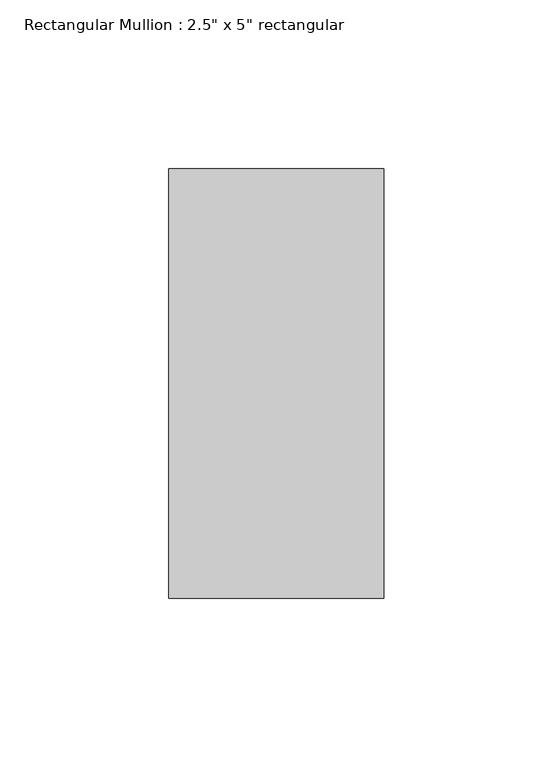
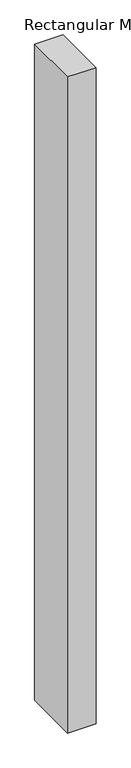
"""IFC4 building model written with IfcOpenShell, lengths in millimetres: member geometry."""

from ifc_helpers import new_model, si_unit, frame, origin, place, context, project, spatial, polyline, outline, extrude, source, transform, mapped, element, save


def member_fedd83b6(model_context):
    return source(origin(), model_context, "Body", "SweptSolid", [
        extrude(outline(polyline([(0.0, 63.5), (0.0, -63.5), (-63.5, -63.5), (-63.5, 63.5), (0.0, 63.5)])), frame((0.0, 0.0, -1549.4), z_axis=(0.0, 0.0, 1.0), x_axis=(1.0, 0.0, 0.0)), (0.0, 0.0, 1.0), 1549.4),
    ])


if __name__ == "__main__":
    model = new_model("IFC4")
    model_context = context("Model", 3, world=origin())
    ifc_project = project(units=[si_unit("LENGTHUNIT", "METRE", prefix="MILLI")], contexts=[model_context])
    site = spatial("IfcSite", under=ifc_project)
    building = spatial("IfcBuilding", under=site)
    placement = place(None, origin())
    member_shape = member_fedd83b6(model_context)
    element("IfcMember", 1, ObjectType="Rectangular Mullion : 2.5\" x 5\" rectangular", at=placement, inside=building, context=model_context, shape_type="MappedRepresentation", body=[
        mapped(member_shape, transform((0.0, 0.0, 0.0), x_axis=(1.0, 0.0, 0.0), y_axis=(0.0, 1.0, 0.0), z_axis=(0.0, 0.0, 1.0))),
    ])
    save(model, "model.ifc")

# Revit data of these elements
# Type "Rectangular Mullion : 2.5\" x 5\" rectangular"
#   built-in parameter 1007304 = 0.416667 (stored number, unit not read)
#   built-in parameter 1007301 = 0.104167 (stored number, unit not read)
#   built-in parameter 1007300 = 0.104167 (stored number, unit not read)
# Element 1 (IfcMember, "Rectangular Mullion : 2.5\" x 5\" rectangular")
#   Materials on its faces: "Iron, Ductile"
# Materials
#   "Iron, Ductile": class "Metal", colour RGB 0 0 0, transparency 0, Description = "Ductile cast iron", Cost = 0
